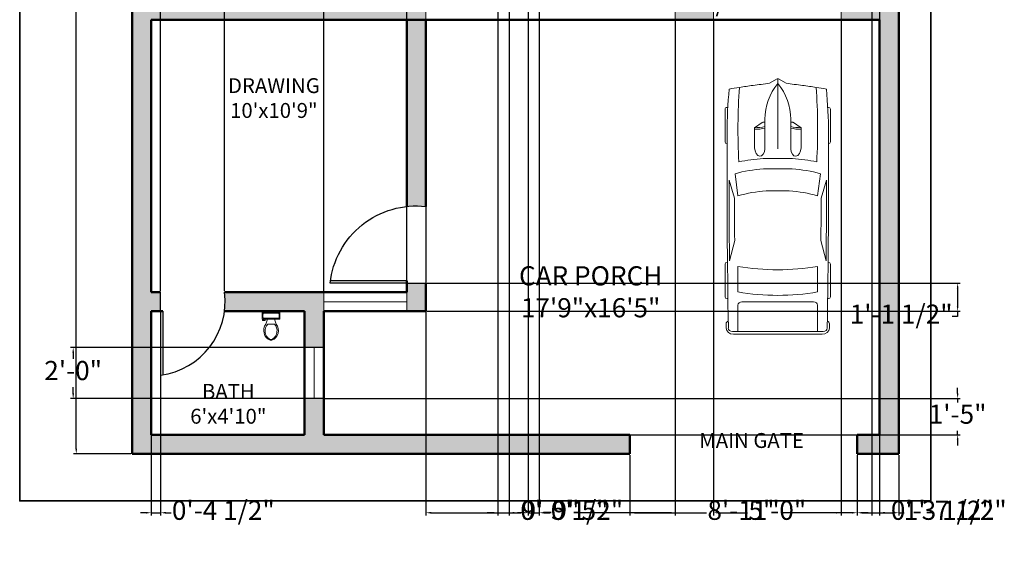
# Model space of a CAD drawing. Units: inches. Extents: x 3695 to 4182, y 4462 to 5050.
# Tile 1 of 3: x 3718 to 4181, y 4462 to 4708. Entities that reach past the tile are written whole.
import ezdxf

# ---------------------------------------------------------------- set-up
doc = ezdxf.new("R2010")
doc.units = ezdxf.units.IN
for name, color, linetype, lineweight in [('A-ANNO-DIMS', 2, 'Continuous', 18), ('A-ANNO-TEXT', 7, 'Continuous', 25), ('A-ANNO-TTLB', 7, 'Continuous', 35), ('A-AREA-IDEN', 7, 'Continuous', 25), ('A-DOOR', 3, 'Continuous', 25), ('A-FLOR-FIXT', 9, 'Continuous', 18), ('A-GLAZ', 4, 'Continuous', 18), ('A-SITE-VEHI', 8, 'Continuous', 13), ('A-WALL', 7, 'Continuous', 50)]:
    doc.layers.add(name, color=color, linetype=linetype, lineweight=lineweight)
doc.layers.add('A-WALL-PATT', color=18, linetype='Continuous', lineweight=13, true_color=0x000000)
doc.styles.get("Standard").update_dxf_attribs({"font": 'arial.ttf'})
doc.dimstyles.new('ISO-25', dxfattribs={"dimtxt": 9, "dimasz": 2.5, "dimexe": 1.25, "dimexo": 0.625, "dimgap": 2, "dimtad": 0, "dimtih": 1, "dimtoh": 1, "dimdec": 1, "dimlunit": 4, "dimtxsty": 'Standard', "dimcen": 2.5, "dimadec": 0, "dimazin": 0, "dimtfac": 0.5, "dimtdec": 1, "dimtmove": 0, "dimatfit": 3, "dimfxl": 1, "dimarcsym": 0})

# ---------------------------------------------------------------- blocks, each defined once
blk = doc.blocks.new('*U5')
for p, q in [((21.1, 37.41), (21.1, 36.83)), ((46.55, 38.89), (22.35, 38.89)), ((47.8, 37.39), (47.8, 37.41)), ((135.45, 37.07), (135.45, 37.41)), ((136.7, 38.89), (160.9, 38.89)), ((162.15, 37.41), (162.15, 36.77)), ((70.03, 31.54), (86.41, 29.35)), ((87.99, 31.87), (74.76, 35.92)), ((134.31, 35.6), (119.29, 31.78)), ((138.42, 29.35), (157.25, 29.35)), ((186.47, 29.35), (167.01, 29.35)), ((186.47, -33.5), (186.47, 33.5)), ((188.4, -32.76), (188.4, 32.76)), ((164.52, 26.39), (164.52, -26.39)), ((32.27, 11.63), (36.13, 17.17)), ((36.13, 17.17), (50.94, 17.17)), ((29.77, 9.51), (51.68, 9.51)), ((32.12, 9.51), (32.12, 11.15)), ((58.92, -10.77), (58.92, 10.77)), ((66.55, -10.53), (66.55, 10.53)), ((82.74, 8.5), (82.74, -8.5)), ((186.47, -10.53), (186.47, 10.53)), ((3.27, 6.13), (0.1, 0.41)), ((0, 0), (51.68, 0)), ((0.1, -0.41), (3.27, -6.13)), ((29.77, -9.51), (51.68, -9.51)), ((32.12, -9.51), (32.12, -11.15)), ((32.27, -11.63), (36.13, -17.17)), ((36.13, -17.17), (50.94, -17.17)), ((86.41, -29.35), (70.03, -31.54)), ((87.99, -31.87), (74.76, -35.92)), ((134.31, -35.6), (119.29, -31.78)), ((157.25, -29.35), (138.42, -29.35)), ((167.01, -29.35), (186.47, -29.35)), ((21.1, -37.41), (21.1, -36.83)), ((46.55, -38.89), (22.35, -38.89)), ((47.8, -37.39), (47.8, -37.41)), ((135.45, -37.07), (135.45, -37.41)), ((136.7, -38.89), (160.9, -38.89)), ((162.15, -37.41), (162.15, -36.77))]:
    blk.add_line(p, q)
for centre, major_axis, ratio, start_param, end_param in [((41.19, -490.86), (0, 528.23), 0.842304, 0.00281, 0.075598), ((22.35, 37.41), (0, -1.48), 0.842304, 3.141593, 4.712389), ((64.48, -10555.62), (0, 10593.03), 0.842304, -0.013397, 0.002797), ((46.55, 37.41), (0, 1.48), 0.842304, -1.570796, 0), ((136.7, 37.41), (0, -1.48), 0.842304, 3.141593, 4.712389), ((160.9, 37.41), (0, 1.48), 0.842304, -1.570796, 0), ((180.63, 35.84), (0, 2.22), 0.842304, -0.013017, 1.249894), ((64.48, -10556.36), (0, 10595.31), 0.842304, -0.013397, -0.013017), ((183.98, 33.5), (0, -2.96), 0.842304, 1.570796, 3.128196), ((183.98, 32.76), (0, -5.25), 0.842304, 1.570796, 3.128196), ((266.03, -27.52), (0, 313.31), 0.842304, 1.367076, 1.39176), ((37.47, -593.96), (0, -623.33), 0.842304, 3.096046, 3.200911), ((135.29, 5.39), (0, 81.77), 0.842304, 1.245306, 1.50788), ((64.48, -10555.62), (0, -10591.55), 0.842304, 3.133765, 3.140441), ((149.6, 2.8), (0, -79.58), 0.842304, 4.372215, 4.640744), ((95.79, -3666.35), (0, -3698.24), 0.842304, 3.134049, 3.144098), ((17.08, 0), (0, 147.02), 0.842304, 4.511394, 4.913384), ((35.91, 0), (0, 147.02), 0.842304, 4.511394, 4.913384), ((167.01, 26.39), (0, 2.96), 0.842304, 0, 1.570796), ((259.18, -27.52), (0, -305.3), 0.842304, 4.528606, 4.561838), ((134.4, 5.39), (0, -89.78), 0.842304, 4.449482, 4.652344), ((-204.49, 52.4), (0, -250.96), 0.842304, 1.385369, 1.434372), ((13.04, 17.01), (0, 27.42), 0.842304, 4.435146, 4.718221), ((14.2, 17.01), (0, 27.42), 0.842304, 4.435146, 4.718221), ((50.79, 13.34), (6.34, -0.36), 0.603834, -1.395552, 1.581315), ((29.77, -46.66), (0, 56.17), 0.842304, 0, 0.590319), ((32.75, 11.15), (0, 0.74), 0.842304, 0.879714, 1.570796), ((0.62, 0), (0, -0.74), 0.842304, 4.131459, 5.293319), ((-204.49, -52.4), (0, 250.96), 0.842304, -1.434372, -1.385369), ((29.77, 46.66), (0, 56.17), 0.842304, 2.551274, 3.141593), ((32.75, -11.15), (0, -0.74), 0.842304, 4.712389, 5.403472), ((13.04, -17.01), (0, -27.42), 0.842304, 1.564964, 1.848039), ((14.2, -17.01), (0, -27.42), 0.842304, 1.564964, 1.848039), ((134.4, -5.39), (0, -89.78), 0.842304, -1.510751, -1.307889), ((135.29, -5.39), (0, -81.77), 0.842304, -1.50788, -1.245306), ((149.6, -2.8), (0, -79.58), 0.842304, -1.499151, -1.230623), ((259.18, 27.52), (0, 305.3), 0.842304, 1.721348, 1.754579), ((266.03, 27.52), (0, 313.31), 0.842304, 1.749832, 1.774517), ((37.47, 593.96), (0, -623.33), 0.842304, -0.059319, 0.045547), ((167.01, -26.39), (0, -2.96), 0.842304, 4.712389, 6.283185), ((41.19, 490.86), (0, -528.23), 0.842304, -0.075598, -0.00281), ((64.48, 10555.62), (0, -10591.55), 0.842304, 0.001152, 0.007828), ((95.79, 3666.35), (0, -3698.24), 0.842304, -0.002505, 0.007544), ((183.98, -33.5), (0, 2.96), 0.842304, 3.15499, 4.712389), ((183.98, -32.76), (0, -5.25), 0.842304, 0.013397, 1.570796), ((22.35, -37.41), (0, 1.48), 0.842304, 1.570796, 3.141593), ((64.48, 10555.62), (0, 10593.03), 0.842304, 3.138796, 3.15499), ((46.55, -37.41), (0, -1.48), 0.842304, 0, 1.570796), ((136.7, -37.41), (0, -1.48), 0.842304, -1.570796, 0), ((160.9, -37.41), (0, 1.48), 0.842304, 3.141593, 4.712389), ((180.63, -35.84), (0, -2.22), 0.842304, -1.249894, 0.013017), ((64.48, 10556.36), (0, 10595.31), 0.842304, 3.15461, 3.15499)]:
    blk.add_ellipse(centre, major_axis=major_axis, ratio=ratio, start_param=start_param, end_param=end_param)
at = {"extrusion": (0, 0, -1)}
blk.add_ellipse((50.79, -13.34), major_axis=(6.34, 0.36), ratio=0.603834, start_param=-1.395552, end_param=1.581315, dxfattribs=at)
blk = doc.blocks.new('*U7')
for p, q in [((-10, -8.5), (-8, -8.5)), ((-10, -9.5), (-10, -8.5)), ((-7, -9.5), (-10, -9.5)), ((-8, -8.5), (-8, -8)), ((-7, -8), (-7, -9.5)), ((-4, -8), (-6, -14)), ((4, -8), (6, -14)), ((9.5, -6), (9.5, -2)), ((4, -14), (-4, -14))]:
    blk.add_line(p, q)
blk.add_lwpolyline([(10.5, -8), (10.5, 0), (-10.5, 0), (-10.5, -8)], close=True)
for points in [[(-9.5, -2), (-9.5, -6)], [(8.5, -1), (-8.5, -1)], [(-8.5, -7), (8.5, -7)]]:
    blk.add_lwpolyline(points)
for centre, radius, start, end in [((-8.6, -1.9), 0.884, 81.8699, 188.1301), ((-8.6, -6.1), 0.884, 171.8699, 278.1301), ((8.6, -1.9), 0.884, 351.8699, 98.1301), ((8.6, -6.1), 0.884, 261.8699, 8.1301), ((3.5, -21.6), 12.2, 141.4691, 247.9714), ((4.2, -21.8), 11.3, 136.3677, 238.9468), ((-3.5, -21.6), 12.2, 292.0284, 38.5307), ((-4.2, -21.8), 11.3, 301.053, 43.6321), ((0, -27.9), 4, 245.7318, 294.2682), ((0, -29), 4, 254.8605, 285.1395)]:
    blk.add_arc(centre, radius, start, end)
blk = doc.blocks.new('*D12')
at = {"layer": 'A-ANNO-DIMS', "color": 0, "lineweight": -2, "transparency": 16777216}
for p, q in [((3770.34, 5007.52), (3743.5, 5007.52)), ((3744.75, 5005.02), (3744.75, 4762.04)), ((3744.75, 4506.02), (3744.75, 4749)), ((3770.34, 4503.52), (3743.5, 4503.52))]:
    blk.add_line(p, q, dxfattribs=at)
at = {"layer": 'A-ANNO-DIMS', "color": 0, "transparency": 16777216}
for points in [[(3744.34, 5005.02), (3745.17, 5005.02), (3744.75, 5007.52)], [(3744.34, 4506.02), (3745.17, 4506.02), (3744.75, 4503.52)]]:
    blk.add_solid(points, dxfattribs=at)
at = {"layer": 'Defpoints', "color": 0, "transparency": 16777216}
for p in [(3770.96, 5007.52), (3744.75, 4503.52), (3770.96, 4503.52)]:
    blk.add_point(p, dxfattribs=at)
at = {"layer": 'A-ANNO-DIMS', "color": 0, "transparency": 16777216, "insert": (3744.75, 4755.52), "char_height": 9, "attachment_point": 5}
blk.add_mtext("42'", dxfattribs=at)
blk = doc.blocks.new('DOOR-SINGLE-36IN')
for p, q in [((35.25, 9), (35.25, 45)), ((36.25, 9), (36.25, 45)), ((36.25, 9), (36.25, 0))]:
    blk.add_line(p, q)
blk.add_arc((40.75, 4.5), 40.75, 96.3402, 186.3402)
blk = doc.blocks.new('*D28')
at = {"layer": 'A-ANNO-DIMS', "color": 0, "lineweight": -2, "transparency": 16777216}
for p, q in [((4067.16, 4728.47), (4063.98, 4728.47)), ((4065.23, 4725.97), (4065.23, 4719.62)), ((4067.16, 4717.12), (4063.98, 4717.12)), ((4065.23, 4717.12), (4065.23, 4714.62)), ((4065.23, 4714.62), (4062.73, 4714.62))]:
    blk.add_line(p, q, dxfattribs=at)
at = {"layer": 'A-ANNO-DIMS', "color": 0, "transparency": 16777216}
for points in [[(4064.81, 4725.97), (4065.65, 4725.97), (4065.23, 4728.47)], [(4064.81, 4719.62), (4065.65, 4719.62), (4065.23, 4717.12)]]:
    blk.add_solid(points, dxfattribs=at)
at = {"layer": 'Defpoints', "color": 0, "transparency": 16777216}
for p in [(4067.78, 4728.47), (4065.23, 4717.12), (4067.78, 4717.12)]:
    blk.add_point(p, dxfattribs=at)
at = {"layer": 'A-ANNO-DIMS', "color": 0, "transparency": 16777216, "insert": (4034.79, 4714.62), "char_height": 9, "attachment_point": 5}
blk.add_mtext('0\'-11 1/2"', dxfattribs=at)
blk = doc.blocks.new('*D31')
at = {"layer": 'A-ANNO-DIMS', "color": 0, "lineweight": -2, "transparency": 16777216}
for p, q in [((4004.7, 4502.9), (4004.7, 4474.62)), ((4111.49, 4502.9), (4111.49, 4474.62)), ((4007.2, 4475.87), (4040.63, 4475.87)), ((4108.99, 4475.87), (4075.56, 4475.87))]:
    blk.add_line(p, q, dxfattribs=at)
at = {"layer": 'A-ANNO-DIMS', "color": 0, "transparency": 16777216}
for points in [[(4007.2, 4476.29), (4007.2, 4475.46), (4004.7, 4475.87)], [(4108.99, 4476.29), (4108.99, 4475.46), (4111.49, 4475.87)]]:
    blk.add_solid(points, dxfattribs=at)
at = {"layer": 'Defpoints', "color": 0, "transparency": 16777216}
for p in [(4004.7, 4503.52), (4111.49, 4503.52), (4111.49, 4475.87)]:
    blk.add_point(p, dxfattribs=at)
at = {"layer": 'A-ANNO-DIMS', "color": 0, "transparency": 16777216, "insert": (4058.09, 4475.87), "char_height": 9, "attachment_point": 5}
blk.add_mtext('8\'-11"', dxfattribs=at)
blk = doc.blocks.new('*D32')
at = {"layer": 'A-ANNO-DIMS', "color": 0, "lineweight": -2, "transparency": 16777216}
for p, q in [((4111.49, 4502.9), (4111.49, 4474.62)), ((4130.96, 4502.9), (4130.96, 4474.62)), ((4113.99, 4475.87), (4128.46, 4475.87)), ((4130.96, 4475.87), (4133.46, 4475.87))]:
    blk.add_line(p, q, dxfattribs=at)
at = {"layer": 'A-ANNO-DIMS', "color": 0, "transparency": 16777216}
for points in [[(4113.99, 4476.29), (4113.99, 4475.46), (4111.49, 4475.87)], [(4128.46, 4476.29), (4128.46, 4475.46), (4130.96, 4475.87)]]:
    blk.add_solid(points, dxfattribs=at)
at = {"layer": 'Defpoints', "color": 0, "transparency": 16777216}
for p in [(4111.49, 4503.52), (4130.96, 4503.52), (4130.96, 4475.87)]:
    blk.add_point(p, dxfattribs=at)
at = {"layer": 'A-ANNO-DIMS', "color": 0, "transparency": 16777216, "insert": (4157.49, 4475.87), "char_height": 9, "attachment_point": 5}
blk.add_mtext('1\'-7 1/2"', dxfattribs=at)
blk = doc.blocks.new('*D34')
at = {"layer": 'A-ANNO-DIMS', "color": 0, "lineweight": -2, "transparency": 16777216}
for p, q in [((3908.96, 4706.9), (3908.96, 4474.62)), ((4025.96, 4706.9), (4025.96, 4474.62)), ((3911.46, 4475.87), (3953.5, 4475.87)), ((4023.46, 4475.87), (3981.43, 4475.87))]:
    blk.add_line(p, q, dxfattribs=at)
at = {"layer": 'A-ANNO-DIMS', "color": 0, "transparency": 16777216}
for points in [[(3911.46, 4476.29), (3911.46, 4475.46), (3908.96, 4475.87)], [(4023.46, 4476.29), (4023.46, 4475.46), (4025.96, 4475.87)]]:
    blk.add_solid(points, dxfattribs=at)
at = {"layer": 'Defpoints', "color": 0, "transparency": 16777216}
for p in [(3908.96, 4707.52), (4025.96, 4707.52), (4025.96, 4475.87)]:
    blk.add_point(p, dxfattribs=at)
at = {"layer": 'A-ANNO-DIMS', "color": 0, "transparency": 16777216, "insert": (3967.46, 4475.87), "char_height": 9, "attachment_point": 5}
blk.add_mtext('9\'-9"', dxfattribs=at)
blk = doc.blocks.new('*D35')
at = {"layer": 'A-ANNO-DIMS', "color": 0, "lineweight": -2, "transparency": 16777216}
for p, q in [((4043.96, 4706.9), (4043.96, 4474.62)), ((4103.96, 4706.9), (4103.96, 4474.62)), ((4046.46, 4475.87), (4060, 4475.87)), ((4101.46, 4475.87), (4087.93, 4475.87))]:
    blk.add_line(p, q, dxfattribs=at)
at = {"layer": 'A-ANNO-DIMS', "color": 0, "transparency": 16777216}
for points in [[(4046.46, 4476.29), (4046.46, 4475.46), (4043.96, 4475.87)], [(4101.46, 4476.29), (4101.46, 4475.46), (4103.96, 4475.87)]]:
    blk.add_solid(points, dxfattribs=at)
at = {"layer": 'Defpoints', "color": 0, "transparency": 16777216}
for p in [(4043.96, 4707.52), (4103.96, 4707.52), (4103.96, 4475.87)]:
    blk.add_point(p, dxfattribs=at)
at = {"layer": 'A-ANNO-DIMS', "color": 0, "transparency": 16777216, "insert": (4073.96, 4475.87), "char_height": 9, "attachment_point": 5}
blk.add_mtext('5\'-0"', dxfattribs=at)
blk = doc.blocks.new('*D36')
at = {"layer": 'A-ANNO-DIMS', "color": 0, "lineweight": -2, "transparency": 16777216}
for p, q in [((3909.59, 4583.78), (4159.86, 4583.78)), ((4158.61, 4581.28), (4158.61, 4573.02)), ((3909.59, 4570.52), (4159.86, 4570.52)), ((4158.61, 4568.02), (4156.11, 4568.02)), ((4158.61, 4570.52), (4158.61, 4568.02))]:
    blk.add_line(p, q, dxfattribs=at)
at = {"layer": 'A-ANNO-DIMS', "color": 0, "transparency": 16777216}
for points in [[(4158.2, 4581.28), (4159.03, 4581.28), (4158.61, 4583.78)], [(4158.2, 4573.02), (4159.03, 4573.02), (4158.61, 4570.52)]]:
    blk.add_solid(points, dxfattribs=at)
at = {"layer": 'Defpoints', "color": 0, "transparency": 16777216}
for p in [(3908.96, 4583.78), (3908.96, 4570.52), (4158.61, 4570.52)]:
    blk.add_point(p, dxfattribs=at)
at = {"layer": 'A-ANNO-DIMS', "color": 0, "transparency": 16777216, "insert": (4132.09, 4568.02), "char_height": 9, "attachment_point": 5}
blk.add_mtext('1\'-1 1/2"', dxfattribs=at)
blk = doc.blocks.new('*D37')
at = {"layer": 'A-ANNO-DIMS', "color": 0, "lineweight": -2, "transparency": 16777216}
for p, q in [((3860.96, 4580.15), (3860.96, 5036.42)), ((3863.46, 5035.17), (3866.51, 5035.17)), ((3897.46, 5035.17), (3894.42, 5035.17)), ((3899.96, 4580.15), (3899.96, 5036.42))]:
    blk.add_line(p, q, dxfattribs=at)
at = {"layer": 'A-ANNO-DIMS', "color": 0, "transparency": 16777216}
for points in [[(3863.46, 5035.59), (3863.46, 5034.76), (3860.96, 5035.17)], [(3897.46, 5035.59), (3897.46, 5034.76), (3899.96, 5035.17)]]:
    blk.add_solid(points, dxfattribs=at)
at = {"layer": 'Defpoints', "color": 0, "transparency": 16777216}
for p in [(3899.96, 5035.17), (3860.96, 4579.52), (3899.96, 4579.52)]:
    blk.add_point(p, dxfattribs=at)
at = {"layer": 'A-ANNO-DIMS', "color": 0, "transparency": 16777216, "insert": (3880.46, 5035.17), "char_height": 9, "attachment_point": 5}
blk.add_mtext('3\'-3"', dxfattribs=at)
blk = doc.blocks.new('*D38')
at = {"layer": 'A-ANNO-DIMS', "color": 0, "lineweight": -2, "transparency": 16777216}
for p, q in [((3860.34, 4553.52), (3742.06, 4553.52)), ((3743.31, 4551.02), (3743.31, 4548.12)), ((3743.31, 4532.02), (3743.31, 4534.93)), ((3860.34, 4529.52), (3742.06, 4529.52))]:
    blk.add_line(p, q, dxfattribs=at)
at = {"layer": 'A-ANNO-DIMS', "color": 0, "transparency": 16777216}
for points in [[(3742.9, 4551.02), (3743.73, 4551.02), (3743.31, 4553.52)], [(3742.9, 4532.02), (3743.73, 4532.02), (3743.31, 4529.52)]]:
    blk.add_solid(points, dxfattribs=at)
at = {"layer": 'Defpoints', "color": 0, "transparency": 16777216}
for p in [(3743.31, 4553.52), (3860.96, 4553.52), (3860.96, 4529.52)]:
    blk.add_point(p, dxfattribs=at)
at = {"layer": 'A-ANNO-DIMS', "color": 0, "transparency": 16777216, "insert": (3743.31, 4541.52), "char_height": 9, "attachment_point": 5}
blk.add_mtext('2\'-0"', dxfattribs=at)
blk = doc.blocks.new('*D39')
at = {"layer": 'A-ANNO-DIMS', "color": 0, "lineweight": -2, "transparency": 16777216}
for p, q in [((4158.61, 4532.02), (4158.61, 4534.52)), ((3861.59, 4529.52), (4159.86, 4529.52)), ((4158.61, 4529.52), (4158.61, 4527.62)), ((3861.59, 4512.52), (4159.86, 4512.52)), ((4158.61, 4512.52), (4158.61, 4514.43)), ((4158.61, 4510.02), (4158.61, 4507.52))]:
    blk.add_line(p, q, dxfattribs=at)
at = {"layer": 'A-ANNO-DIMS', "color": 0, "transparency": 16777216}
for points in [[(4158.2, 4532.02), (4159.03, 4532.02), (4158.61, 4529.52)], [(4158.2, 4510.02), (4159.03, 4510.02), (4158.61, 4512.52)]]:
    blk.add_solid(points, dxfattribs=at)
at = {"layer": 'Defpoints', "color": 0, "transparency": 16777216}
for p in [(3860.96, 4529.52), (4158.61, 4529.52), (3860.96, 4512.52)]:
    blk.add_point(p, dxfattribs=at)
at = {"layer": 'A-ANNO-DIMS', "color": 0, "transparency": 16777216, "insert": (4158.61, 4521.02), "char_height": 9, "attachment_point": 5}
blk.add_mtext('1\'-5"', dxfattribs=at)
blk = doc.blocks.new('*D41')
at = {"layer": 'A-ANNO-DIMS', "color": 0, "lineweight": -2, "transparency": 16777216}
for p, q in [((3956.96, 4802.9), (3956.96, 4474.62)), ((3962.16, 4802.9), (3962.16, 4474.62)), ((3954.46, 4475.87), (3951.96, 4475.87)), ((3956.96, 4475.87), (3962.16, 4475.87)), ((3964.66, 4475.87), (3967.16, 4475.87))]:
    blk.add_line(p, q, dxfattribs=at)
at = {"layer": 'A-ANNO-DIMS', "color": 0, "transparency": 16777216}
for points in [[(3954.46, 4476.29), (3954.46, 4475.46), (3956.96, 4475.87)], [(3964.66, 4476.29), (3964.66, 4475.46), (3962.16, 4475.87)]]:
    blk.add_solid(points, dxfattribs=at)
at = {"layer": 'Defpoints', "color": 0, "transparency": 16777216}
for p in [(3956.96, 4803.52), (3962.16, 4803.52), (3962.16, 4475.87)]:
    blk.add_point(p, dxfattribs=at)
at = {"layer": 'A-ANNO-DIMS', "color": 0, "transparency": 16777216, "insert": (3981.12, 4475.87), "char_height": 9, "attachment_point": 5}
blk.add_mtext('0\'-5"', dxfattribs=at)
blk = doc.blocks.new('*D42')
at = {"layer": 'A-ANNO-DIMS', "color": 0, "lineweight": -2, "transparency": 16777216}
for p, q in [((3942.69, 4837.4), (3942.69, 4474.62)), ((3947.96, 4837.4), (3947.96, 4474.62)), ((3940.19, 4475.87), (3937.69, 4475.87)), ((3942.69, 4475.87), (3947.96, 4475.87)), ((3950.46, 4475.87), (3952.96, 4475.87))]:
    blk.add_line(p, q, dxfattribs=at)
at = {"layer": 'A-ANNO-DIMS', "color": 0, "transparency": 16777216}
for points in [[(3940.19, 4476.29), (3940.19, 4475.46), (3942.69, 4475.87)], [(3950.46, 4476.29), (3950.46, 4475.46), (3947.96, 4475.87)]]:
    blk.add_solid(points, dxfattribs=at)
at = {"layer": 'Defpoints', "color": 0, "transparency": 16777216}
for p in [(3942.69, 4838.02), (3947.96, 4838.02), (3947.96, 4475.87)]:
    blk.add_point(p, dxfattribs=at)
at = {"layer": 'A-ANNO-DIMS', "color": 0, "transparency": 16777216, "insert": (3977.41, 4475.87), "char_height": 9, "attachment_point": 5}
blk.add_mtext('0\'-5 1/2"', dxfattribs=at)
blk = doc.blocks.new('*D45')
at = {"layer": 'A-ANNO-DIMS', "color": 0, "lineweight": -2, "transparency": 16777216}
for p, q in [((3781.88, 5035.17), (3779.38, 5035.17)), ((3784.38, 4580.15), (3784.38, 5036.42)), ((3784.38, 5035.17), (3785.34, 5035.17)), ((3814.38, 5035.17), (3813.42, 5035.17)), ((3814.38, 4580.15), (3814.38, 5036.42)), ((3816.88, 5035.17), (3819.38, 5035.17))]:
    blk.add_line(p, q, dxfattribs=at)
at = {"layer": 'A-ANNO-DIMS', "color": 0, "transparency": 16777216}
for points in [[(3781.88, 5035.59), (3781.88, 5034.76), (3784.38, 5035.17)], [(3816.88, 5035.59), (3816.88, 5034.76), (3814.38, 5035.17)]]:
    blk.add_solid(points, dxfattribs=at)
at = {"layer": 'Defpoints', "color": 0, "transparency": 16777216}
for p in [(3814.38, 5035.17), (3784.38, 4579.52), (3814.38, 4579.52)]:
    blk.add_point(p, dxfattribs=at)
at = {"layer": 'A-ANNO-DIMS', "color": 0, "transparency": 16777216, "insert": (3799.38, 5035.17), "char_height": 9, "attachment_point": 5}
blk.add_mtext('2\'-6"', dxfattribs=at)
blk = doc.blocks.new('*D50')
at = {"layer": 'A-ANNO-DIMS', "color": 0, "lineweight": -2, "transparency": 16777216}
for p, q in [((4118.4, 4931.9), (4118.4, 4474.62)), ((4121.96, 4931.9), (4121.96, 4474.62)), ((4115.9, 4475.87), (4113.4, 4475.87)), ((4118.4, 4475.87), (4121.96, 4475.87)), ((4124.46, 4475.87), (4126.96, 4475.87))]:
    blk.add_line(p, q, dxfattribs=at)
at = {"layer": 'A-ANNO-DIMS', "color": 0, "transparency": 16777216}
for points in [[(4115.9, 4476.29), (4115.9, 4475.46), (4118.4, 4475.87)], [(4124.46, 4476.29), (4124.46, 4475.46), (4121.96, 4475.87)]]:
    blk.add_solid(points, dxfattribs=at)
at = {"layer": 'Defpoints', "color": 0, "transparency": 16777216}
for p in [(4118.4, 4932.52), (4121.96, 4932.52), (4121.96, 4475.87)]:
    blk.add_point(p, dxfattribs=at)
at = {"layer": 'A-ANNO-DIMS', "color": 0, "transparency": 16777216, "insert": (4151.41, 4475.87), "char_height": 9, "attachment_point": 5}
blk.add_mtext('0\'-3 1/2"', dxfattribs=at)
blk = doc.blocks.new('*D51')
at = {"layer": 'A-ANNO-DIMS', "color": 0, "lineweight": -2, "transparency": 16777216}
for p, q in [((3779.96, 4569.9), (3779.96, 4474.62)), ((3784.38, 4569.9), (3784.38, 4474.62)), ((3777.46, 4475.87), (3774.96, 4475.87)), ((3779.96, 4475.87), (3784.38, 4475.87)), ((3786.88, 4475.87), (3789.38, 4475.87))]:
    blk.add_line(p, q, dxfattribs=at)
at = {"layer": 'A-ANNO-DIMS', "color": 0, "transparency": 16777216}
for points in [[(3777.46, 4476.29), (3777.46, 4475.46), (3779.96, 4475.87)], [(3786.88, 4476.29), (3786.88, 4475.46), (3784.38, 4475.87)]]:
    blk.add_solid(points, dxfattribs=at)
at = {"layer": 'Defpoints', "color": 0, "transparency": 16777216}
for p in [(3779.96, 4570.52), (3784.38, 4570.52), (3784.38, 4475.87)]:
    blk.add_point(p, dxfattribs=at)
at = {"layer": 'A-ANNO-DIMS', "color": 0, "transparency": 16777216, "insert": (3813.83, 4475.87), "char_height": 9, "attachment_point": 5}
blk.add_mtext('0\'-4 1/2"', dxfattribs=at)
blk = doc.blocks.new('*D53')
at = {"layer": 'A-ANNO-DIMS', "color": 0, "lineweight": -2, "transparency": 16777216}
for p, q in [((3829.71, 4800.29), (3829.71, 4748.1)), ((3829.71, 4716.79), (3829.71, 4745.6)), ((3832.21, 4716.79), (3829.71, 4716.79))]:
    blk.add_line(p, q, dxfattribs=at)
at = {"layer": 'A-ANNO-DIMS', "color": 0, "transparency": 16777216}
blk.add_solid([(3830.13, 4745.6), (3829.29, 4745.6), (3829.71, 4748.1)], dxfattribs=at)
at = {"layer": 'Defpoints', "color": 0, "transparency": 16777216}
for p in [(3829.71, 4800.29), (3829.71, 4748.1)]:
    blk.add_point(p, dxfattribs=at)
at = {"layer": 'A-ANNO-DIMS', "color": 0, "transparency": 16777216, "insert": (3860.15, 4716.79), "char_height": 9, "attachment_point": 5}
blk.add_mtext('3X R4\'-4"', dxfattribs=at)

msp = doc.modelspace()

# ---------------------------------------------------------------- hatches: boundary and pattern name
at = {"layer": 'A-WALL-PATT'}
h = msp.add_hatch(color=256, dxfattribs=at)
h.dxf.hatch_style = 1
h.paths.add_polyline_path([(3906.69, 4838.02), (3779.96, 4838.02), (3779.96, 4998.52), (3947.96, 4998.52), (3947.96, 4994.14), (3956.96, 4994.14), (3956.96, 4998.52), (4016.96, 4998.52), (4016.96, 4994.14), (4025.96, 4994.14), (4025.96, 4998.52), (4121.96, 4998.52), (4121.96, 4938.52), (4118.4, 4938.52), (4118.4, 4932.52), (4121.96, 4932.52), (4121.96, 4812.52), (4025.96, 4812.52), (3998.16, 4812.52, -0.055385), (3998.16, 4803.52), (4025.96, 4803.52), (4025.96, 4800.38), (4034.96, 4800.38), (4034.96, 4803.52), (4121.96, 4803.52), (4121.96, 4716.52), (4103.96, 4716.52), (4103.96, 4707.52), (4121.96, 4707.52), (4121.96, 4512.52), (4111.49, 4512.52), (4111.49, 4503.52), (4130.96, 4503.52), (4130.96, 5007.52), (3770.96, 5007.52), (3770.96, 4503.52), (4004.7, 4503.52), (4004.7, 4512.52), (3860.96, 4512.52), (3860.96, 4529.52), (3851.96, 4529.52), (3851.96, 4512.52), (3779.96, 4512.52), (3779.96, 4570.52), (3784.38, 4570.52), (3784.38, 4579.52), (3779.96, 4579.52), (3779.96, 4707.52), (3908.96, 4707.52), (3908.96, 4716.52), (3779.96, 4716.52), (3779.96, 4829.02), (3906.69, 4829.02, -0.055385)])
h.paths.add_polyline_path([(4034.96, 4764.38, -0.055385), (4025.96, 4764.38), (4025.96, 4716.52), (4025.96, 4707.52), (4043.96, 4707.52), (4043.96, 4716.52), (4034.96, 4716.52)], flags=17)
h = msp.add_hatch(color=256, dxfattribs=at)
h.dxf.hatch_style = 1
h.paths.add_polyline_path([(3860.96, 4579.52), (3851.96, 4579.52), (3814.38, 4579.52, -0.064942), (3814.38, 4570.52), (3851.96, 4570.52), (3851.96, 4553.52), (3860.96, 4553.52), (3860.96, 4570.52)], flags=17)
h.paths.add_polyline_path([(3908.96, 4707.52), (3899.96, 4707.52), (3899.96, 4619.78, -0.055385), (3908.96, 4619.78)], flags=17)
h = msp.add_hatch(color=256, dxfattribs=at)
h.dxf.hatch_style = 1
h.paths.add_polyline_path([(3908.96, 4579.52), (3908.96, 4583.78), (3899.96, 4583.78), (3899.96, 4579.52), (3899.96, 4570.52), (3908.96, 4570.52)])

# ---------------------------------------------------------------- linework, layer by layer
at = {"layer": 'A-ANNO-TTLB'}
msp.add_lwpolyline([(3718.2, 5049.57), (4146.02, 5049.57), (4146.02, 4481.47), (3718.2, 4481.47)], close=True, dxfattribs=at)
at = {"layer": 'A-DOOR'}
for p, q in [((3784.38, 4570.52), (3784.38, 4579.52)), ((3784.38, 4570.52), (3784.38, 4540.52)), ((3785.38, 4570.52), (3785.38, 4540.52))]:
    msp.add_line(p, q, dxfattribs=at)
msp.add_arc((3779.88, 4575.02), 34.79, 277.4314, 7.4314, dxfattribs=at)
at = {"layer": 'A-GLAZ'}
for p, q in [((3908.96, 4707.52), (3908.96, 4716.52)), ((4025.96, 4716.52), (4025.96, 4707.52)), ((4043.96, 4707.52), (4043.96, 4716.52)), ((4043.96, 4716.52), (4043.96, 4707.52)), ((4103.96, 4707.52), (4103.96, 4716.52)), ((3860.96, 4570.52), (3860.96, 4579.52)), ((3899.96, 4579.52), (3899.96, 4570.52)), ((3860.96, 4575.02), (3899.96, 4575.02)), ((3851.96, 4553.52), (3860.96, 4553.52)), ((3856.46, 4553.52), (3856.46, 4529.52)), ((3851.96, 4529.52), (3860.96, 4529.52))]:
    msp.add_line(p, q, dxfattribs=at)
at = {"layer": 'A-WALL'}
for p, q in [((3770.96, 4503.52), (3770.96, 5007.52)), ((4130.96, 5007.52), (4130.96, 4503.52)), ((4121.96, 4707.52), (3779.96, 4707.52)), ((3779.96, 4579.52), (3779.96, 4707.52)), ((4025.96, 4707.52), (3860.96, 4707.52)), ((3899.96, 4619.78), (3899.96, 4707.52)), ((3908.96, 4619.78), (3908.96, 4707.52)), ((4025.96, 4707.52), (4121.96, 4707.52)), ((4121.96, 4707.52), (4121.96, 4512.52)), ((3899.96, 4579.52), (3899.96, 4584.78)), ((3908.96, 4579.52), (3908.96, 4583.78)), ((3784.38, 4579.52), (3779.96, 4579.52)), ((3851.96, 4579.52), (3814.38, 4579.52)), ((3851.96, 4579.52), (3860.96, 4579.52)), ((3860.96, 4579.52), (3899.96, 4579.52)), ((3908.96, 4579.52), (3908.96, 4570.52)), ((3779.96, 4512.52), (3779.96, 4570.52)), ((3785.38, 4570.52), (3779.96, 4570.52)), ((3851.96, 4570.52), (3814.38, 4570.52)), ((3851.96, 4512.52), (3851.96, 4570.52)), ((3860.96, 4512.52), (3860.96, 4570.52)), ((3860.96, 4570.52), (3908.96, 4570.52)), ((3851.96, 4512.52), (3779.96, 4512.52)), ((4004.7, 4512.52), (3860.96, 4512.52)), ((4004.7, 4512.52), (3956.96, 4512.52)), ((4004.7, 4512.52), (4004.7, 4503.52)), ((4121.96, 4512.52), (4111.49, 4512.52)), ((4121.96, 4512.52), (4111.49, 4512.52)), ((4111.49, 4512.52), (4111.49, 4503.52)), ((4004.7, 4503.52), (3770.96, 4503.52)), ((4130.96, 4503.52), (4111.49, 4503.52))]:
    msp.add_line(p, q, dxfattribs=at)

# ---------------------------------------------------------------- block references
at = {"layer": 'A-DOOR', "extrusion": (0, 0, -1), "zscale": -1, "rotation": 270.0000000000003}
msp.add_blockref('DOOR-SINGLE-36IN', (-3908.96, 4620.03), dxfattribs=at)
at = {"layer": 'A-FLOR-FIXT', "xscale": 0.3973700613755364, "yscale": 0.3973700613755364, "zscale": 0.3973700613755364}
msp.add_blockref('*U7', (3836.22, 4570.02), dxfattribs=at)
at = {"layer": 'A-SITE-VEHI', "xscale": 0.637028620551503, "yscale": 0.637028620551503, "zscale": 0.637028620551503, "rotation": 270}
msp.add_blockref('*U5', (4074.17, 4679.78), dxfattribs=at)

# ---------------------------------------------------------------- texts
at = {"layer": 'A-ANNO-TEXT', "insert": (4022.97, 4513.32), "char_height": 7, "attachment_point": 1}
msp.add_mtext_dynamic_manual_height_columns('\\pxqc;{\\fArial|b1|i0|c0|p34;MAIN GATE}', width=77.7715, gutter_width=12.5, heights=[0], dxfattribs=at)
at = {"layer": 'A-AREA-IDEN', "attachment_point": 1}
for s, width, insert, char_height in [('\\pxqc;{\\fArial|b1|i0|c0|p34;DRAWING\\P10\'x10\'9"}', 103.4114, (3785.84, 4680.04), 7), ('\\pxqc;{\\fArial|b1|i0|c0|p34;CAR PORCH\\P17\'9"x16\'5"}', 98.6697, (3936.97, 4591.69), 9), ('\\pxqc;{\\fArial|b1|i0|c0|p34;BATH\\P6\'x4\'10"}', 65.1341, (3783.61, 4536.39), 7)]:
    msp.add_mtext_dynamic_manual_height_columns(s, width=width, gutter_width=12.5, heights=[0], dxfattribs=dict(at, insert=insert, char_height=char_height))

# ---------------------------------------------------------------- dimensions: what is measured, and where the dimension line sits
at = {"layer": 'A-ANNO-DIMS'}
for base, p1, p2, picture, middle in [((3814.38, 5035.17), (3784.38, 4579.52), (3814.38, 4579.52), '*D45', (3799.38, 5035.17)), ((3899.96, 5035.17), (3860.96, 4579.52), (3899.96, 4579.52), '*D37', (3880.46, 5035.17)), ((4121.96, 4475.87), (4118.4, 4932.52), (4121.96, 4932.52), '*D50', (4151.41, 4475.87)), ((3947.96, 4475.87), (3942.69, 4838.02), (3947.96, 4838.02), '*D42', (3977.41, 4475.87)), ((3962.16, 4475.87), (3956.96, 4803.52), (3962.16, 4803.52), '*D41', (3981.12, 4475.87)), ((4025.96, 4475.87), (3908.96, 4707.52), (4025.96, 4707.52), '*D34', (3967.46, 4475.87)), ((4103.96, 4475.87), (4043.96, 4707.52), (4103.96, 4707.52), '*D35', (4073.96, 4475.87)), ((3784.38, 4475.87), (3779.96, 4570.52), (3784.38, 4570.52), '*D51', (3813.83, 4475.87)), ((4111.49, 4475.87), (4004.7, 4503.52), (4111.49, 4503.52), '*D31', (4058.09, 4475.87)), ((4130.96, 4475.87), (4111.49, 4503.52), (4130.96, 4503.52), '*D32', (4157.49, 4475.87))]:
    dim = msp.add_linear_dim(base=base, p1=p1, p2=p2, dimstyle='ISO-25', override={"dimdec": 1, "dimlfac": 1, "dimrnd": 0, "dimzin": 1, "dimdsep": 46, "dimlunit": 4, "dimfrac": 2}, dxfattribs=at)
    dim.commit()
    dim.dimension.update_dxf_attribs({"geometry": picture, "text_midpoint": middle})
for base, p1, p2, angle, override, picture, middle in [((3744.75, 4503.52), (3770.96, 5007.52), (3770.96, 4503.52), 90, {"dimclrd": 0, "dimclre": 0, "dimclrt": 0}, '*D12', (3744.75, 4755.52)), ((4065.2299, 4717.1184), (4067.7843, 4728.4712), (4067.7843, 4717.1184), 270, {"dimdec": 1, "dimlfac": 1, "dimrnd": 0, "dimzin": 1, "dimdsep": 46, "dimlunit": 4, "dimfrac": 2}, '*D28', (4034.7859, 4714.6184)), ((4158.61, 4570.52), (3908.96, 4583.78), (3908.96, 4570.52), 90, {"dimdec": 1, "dimlfac": 1, "dimrnd": 0, "dimzin": 1, "dimdsep": 46, "dimlunit": 4, "dimfrac": 2}, '*D36', (4132.09, 4568.02)), ((3743.31, 4553.52), (3860.96, 4529.52), (3860.96, 4553.52), 90, {"dimdec": 1, "dimlfac": 1, "dimrnd": 0, "dimzin": 1, "dimdsep": 46, "dimlunit": 4, "dimfrac": 2}, '*D38', (3743.31, 4541.52)), ((4158.61, 4529.52), (3860.96, 4512.52), (3860.96, 4529.52), 90, {"dimdec": 1, "dimlfac": 1, "dimrnd": 0, "dimzin": 1, "dimdsep": 46, "dimlunit": 4, "dimfrac": 2}, '*D39', (4158.61, 4521.02))]:
    dim = msp.add_linear_dim(base=base, p1=p1, p2=p2, angle=angle, dimstyle='ISO-25', override=override, dxfattribs=at)
    dim.commit()
    dim.dimension.update_dxf_attribs({"geometry": picture, "text_midpoint": middle})
dim = msp.add_radius_dim(center=(3829.71, 4800.29), mpoint=(3829.71, 4748.1), text='3X <>', dimstyle='ISO-25', override={"dimdec": 1, "dimlfac": 1, "dimrnd": 0, "dimzin": 1, "dimdsep": 46, "dimlunit": 4, "dimfrac": 2}, dxfattribs=at)
dim.commit()
dim.dimension.update_dxf_attribs({"geometry": '*D53', "text_midpoint": (3860.15, 4716.79), "dimtype": 164})

doc.saveas('drawing.dxf')
